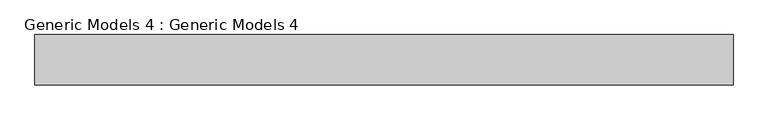
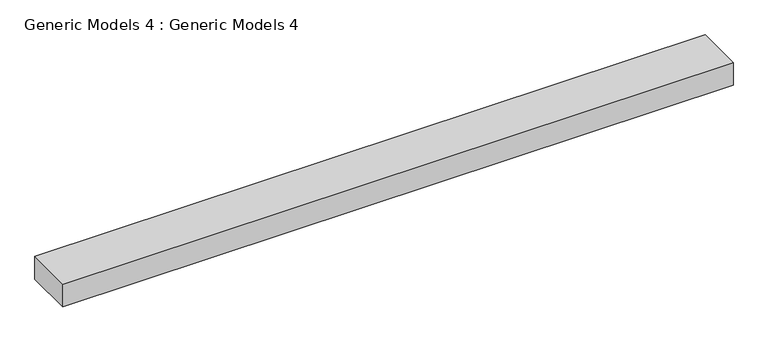
"""IFC4 building model written with IfcOpenShell, lengths in millimetres: proxy geometry, Generic Models 4 : Generic Models 4."""

from ifc_helpers import new_model, si_unit, frame, origin, place, context, project, spatial, polyline, outline, extrude, source, transform, mapped, element, save


def generic_models_4_generic_models_4_4e8aec35(model_context):
    return source(origin(), model_context, "Body", "SweptSolid", [
        extrude(outline(polyline([(-5062.4656154, -4923.9499125), (-9299.6237019, -4923.9499125), (-9299.6237019, -4619.1499125), (-5062.4656154, -4619.1499125), (-5062.4656154, -4923.9499125)])), frame((0.0, 0.0, 5181.6), z_axis=(0.0, 0.0, 1.0), x_axis=(1.0, 0.0, 0.0)), (0.0, 0.0, 1.0), 152.4),
    ])


if __name__ == "__main__":
    model = new_model("IFC4")
    model_context = context("Model", 3, world=origin())
    ifc_project = project(units=[si_unit("LENGTHUNIT", "METRE", prefix="MILLI")], contexts=[model_context])
    site = spatial("IfcSite", under=ifc_project)
    building = spatial("IfcBuilding", under=site)
    placement = place(None, origin())
    generic_models_4_generic_models_4_shape = generic_models_4_generic_models_4_4e8aec35(model_context)
    element("IfcBuildingElementProxy", 1, Name="Generic Models 4 : Generic Models 4", ObjectType="Generic Models 4 : Generic Models 4", at=placement, inside=building, context=model_context, shape_type="MappedRepresentation", body=[
        mapped(generic_models_4_generic_models_4_shape, transform((0.0, 0.0, 0.0), x_axis=(1.0, 0.0, 0.0), y_axis=(0.0, 1.0, 0.0), z_axis=(0.0, 0.0, 1.0))),
    ])
    save(model, "model.ifc")

# Revit data of these elements
# Element 1 (IfcBuildingElementProxy, "Generic Models 4 : Generic Models 4")
#   Materials on its faces: "LIGHT BEIGE"
# Materials
#   "LIGHT BEIGE": class "Generic", colour RGB 120 120 120, transparency 0, Cost = 0
